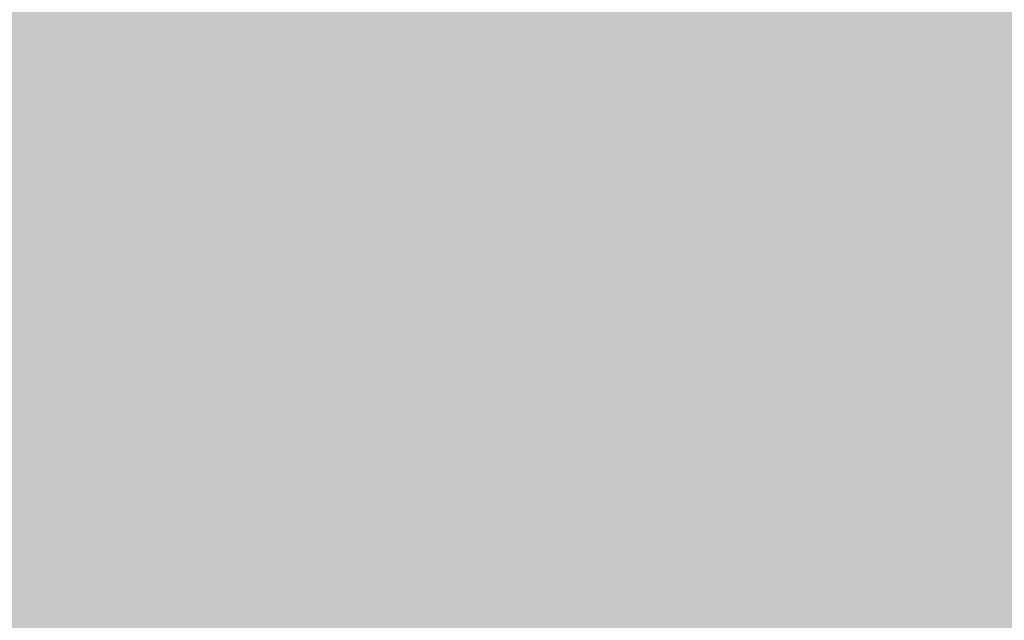
# Model space of a CAD drawing. Units: feet. Extents: x 3168 to 4724, y 827 to 1477.
# Tile 85 of 256: x 3274.148 to 3275.224, y 1098.344 to 1099.001. Entities that reach past the tile are written whole.
import ezdxf

# ---------------------------------------------------------------- set-up
doc = ezdxf.new("R2010")
doc.units = ezdxf.units.FT
doc.layers.add('A-ELEV', color=7, linetype='Continuous', lineweight=35)
doc.layers.add('A-ELEV-PATT', color=8, linetype='Continuous', lineweight=13)

msp = doc.modelspace()

# ---------------------------------------------------------------- hatches: boundary and pattern name
at = {"layer": 'A-ELEV-PATT'}
h = msp.add_hatch(color=256, dxfattribs=at)
h.dxf.hatch_style = 1
edge = h.paths.add_edge_path()
edge.add_ellipse((3552.9058, 979.2201), major_axis=(36.7449, 0), ratio=0.4848485, start_angle=0, end_angle=360)
edge = h.paths.add_edge_path()
edge.add_ellipse((3559.8916, 929.2523), major_axis=(36.7449, 0), ratio=0.4848485, start_angle=0, end_angle=360)
edge = h.paths.add_edge_path()
edge.add_line((3299.3168, 1198.6061), (3479.9167, 1198.6061))
edge.add_line((3479.9167, 1198.6061), (3479.9167, 1209.8686))
edge.add_spline(control_points=[(3479.9167, 1209.8686), (3464.3012, 1209.8686), (3448.6856, 1209.8686), (3410.9491, 1209.8686), (3388.8282, 1209.8686), (3355.6469, 1209.8686), (3344.5864, 1209.8686), (3327.9957, 1209.8686), (3322.4655, 1209.8686), (3314.1702, 1209.8686), (3311.4051, 1209.8686), (3307.2574, 1209.8686), (3305.8748, 1209.8686), (3303.801, 1209.8686), (3303.1097, 1209.8686), (3302.0728, 1209.8686), (3301.7272, 1209.8686), (3301.2087, 1209.8686), (3301.0359, 1209.8686), (3300.7767, 1209.8686), (3300.6903, 1209.8686), (3300.5606, 1209.8686), (3300.5174, 1209.8686), (3300.4526, 1209.8686), (3300.431, 1209.8686), (3300.3986, 1209.8686), (3300.3878, 1209.8686), (3300.3662, 1209.8686), (3300.3457, 1209.8686), (3300.3455, 1209.8686), (3300.3455, 1209.8686), (3300.3433, 1209.8686), (3300.3411, 1209.8686), (3300.3379, 1209.8686), (3300.3368, 1209.8686), (3300.3339, 1209.8686), (3300.3321, 1209.8686), (3300.3255, 1209.8686), (3300.3207, 1209.8686), (3300.3109, 1209.8686), (3300.306, 1209.8686), (3300.2905, 1209.8686), (3300.28, 1209.8686), (3300.2324, 1209.8688), (3300.1953, 1209.869), (3299.9511, 1209.8706), (3299.7448, 1209.8743), (3299.4368, 1209.8833), (3299.3344, 1209.8868), (3299.1811, 1209.8929), (3299.13, 1209.8951), (3298.6522, 1209.9168), (3298.2295, 1209.9457), (3297.6016, 1210.0024), (3297.3934, 1210.0235), (3297.0827, 1210.0583), (3296.9793, 1210.0705), (3296.293, 1210.1549), (3295.7181, 1210.2434), (3294.8687, 1210.3989), (3294.5877, 1210.4545), (3294.1693, 1210.5433), (3294.0304, 1210.5739), (3291.7071, 1211.1012), (3289.6536, 1211.8134), (3285.7763, 1213.564), (3283.9514, 1214.6035), (3280.5122, 1216.9801), (3278.8972, 1218.3176), (3276.3799, 1220.8295), (3275.416, 1221.9177), (3274.0393, 1223.7077), (3273.581, 1224.3495), (3273.1432, 1225.0163)], knot_values=[39.119033, 39.119033, 39.119033, 39.119033, 39.286353, 39.286353, 39.523379, 39.523379, 39.641892, 39.641892, 39.701148, 39.701148, 39.730777, 39.730777, 39.745591, 39.745591, 39.752998, 39.752998, 39.756701, 39.756701, 39.758553, 39.758553, 39.759479, 39.759479, 39.759942, 39.759942, 39.760173, 39.760173, 39.760289, 39.760289, 39.760405, 39.760405, 39.760463, 39.760463, 39.763389, 39.763389, 39.764851, 39.764851, 39.767304, 39.767304, 39.773825, 39.773825, 39.78057, 39.78057, 39.79477, 39.79477, 39.845194, 39.845194, 40.126715, 40.126715, 40.267476, 40.267476, 40.337856, 40.337856, 40.927023, 40.927023, 41.221606, 41.221606, 41.368898, 41.368898, 42.202622, 42.202622, 42.619485, 42.619485, 42.827916, 42.827916, 46.118323, 46.118323, 49.408731, 49.408731, 52.699139, 52.699139, 54.927489, 54.927489, 56.104228, 56.104228, 56.104228, 56.104228], weights=[1, 1, 1, 1, 1, 1, 1, 1, 1, 1, 1, 1, 1, 1, 1, 1, 1, 1, 1, 1, 1, 1, 1, 1, 1, 1, 1, 1, 1, 1, 1, 1, 1, 1, 1, 1, 1, 1, 1, 1, 1, 1, 1, 1, 1, 1, 1, 1, 1, 1, 1, 1, 1, 1, 1, 1, 1, 1, 1, 1, 1, 1, 1, 1, 1, 1, 1, 1, 1, 1, 1, 1, 1, 1], degree=3, periodic=0)
edge.add_line((3273.1432, 1225.0163), (3273.1432, 1099.0163))
edge.add_line((3273.1432, 1099.0163), (3299.3168, 1099.0163))
edge.add_line((3299.3168, 1099.0163), (3299.3168, 1198.6061))
edge = h.paths.add_edge_path()
edge.add_line((3304.7584, 1324.1581), (3479.9167, 1324.1581))
edge.add_line((3479.9167, 1324.1581), (3479.9167, 1335.7146))
edge.add_line((3479.9167, 1335.7146), (3269.1616, 1335.7146))
edge.add_spline(control_points=[(3269.1616, 1335.7146), (3264.0242, 1335.7146), (3258.3641, 1328.9582), (3259.2643, 1323.9003)], knot_values=[0, 0, 0, 0, 15.412191, 15.412191, 15.412191, 15.412191], degree=3, periodic=0)
edge.add_line((3259.2643, 1323.9003), (3265.5168, 1288.7691))
edge.add_line((3265.5168, 1288.7691), (3275.2651, 1261.5456))
edge.add_line((3275.2651, 1261.5456), (3304.7584, 1261.5456))
edge.add_line((3304.7584, 1261.5456), (3304.7584, 1324.1581))
h = msp.add_hatch(color=256, dxfattribs=at)
h.dxf.hatch_style = 1
h.paths.add_polyline_path([(3384.5252, 1099.0163), (3335.0292, 1099.0163), (3299.3168, 1099.0163), (3273.1432, 1099.0163), (3217.5654, 1099.0163), (3168.0693, 827.1163), (3335.0292, 827.1163)])

# ---------------------------------------------------------------- linework, layer by layer
at = {"layer": 'A-ELEV'}
msp.add_open_spline([(3808.5202, 1099.0163), (3808.5202, 1141.4132), (3808.5202, 1183.8102), (3808.5202, 1226.6353), (3808.5202, 1227.0636), (3808.5202, 1227.4918), (3811.4919, 1248.9947), (3814.4635, 1270.4975), (3817.4652, 1292.2176), (3817.4952, 1292.4348), (3817.5253, 1292.652), (3817.5728, 1310.1067), (3817.6203, 1327.5615), (3817.6679, 1345.0163), (3817.6679, 1345.458), (3817.6679, 1345.8996), (3817.6679, 1346.456), (3817.6679, 1346.5708), (3817.6679, 1346.7529), (3817.6679, 1346.8201), (3817.6679, 1346.9349), (3817.6679, 1346.9823), (3817.6679, 1347.0386), (3817.6679, 1347.0474), (3817.6679, 1347.0737), (3817.6679, 1347.0593), (3817.6679, 1347.0615), (3817.6679, 1347.0627), (3817.6679, 1347.066), (3817.6679, 1347.0683), (3817.6679, 1347.075), (3817.6679, 1347.0795), (3817.6678, 1347.0929), (3817.6678, 1347.1019), (3817.6678, 1347.1288), (3817.6677, 1347.1467), (3817.6674, 1347.2004), (3817.6672, 1347.2362), (3817.6661, 1347.3434), (3817.665, 1347.4147), (3817.6608, 1347.6281), (3817.6566, 1347.7697), (3817.64, 1348.1925), (3817.6235, 1348.4716), (3817.5591, 1349.3001), (3817.4961, 1349.8406), (3817.2554, 1351.4242), (3817.0263, 1352.4288), (3816.3069, 1354.8889), (3815.7437, 1356.2687), (3814.464, 1358.8192), (3813.7464, 1359.991), (3812.1958, 1362.1723), (3811.3622, 1363.1821), (3809.5888, 1365.069), (3808.6488, 1365.9461), (3806.6543, 1367.5796), (3805.5997, 1368.3362), (3803.3529, 1369.7223), (3802.1605, 1370.3524), (3799.6008, 1371.4536), (3798.2327, 1371.9255), (3795.2801, 1372.6346), (3793.6931, 1372.8721), (3791.8694, 1372.9265), (3791.7409, 1372.9292), (3791.3534, 1372.9341), (3791.0927, 1372.9329), (3790.3041, 1372.9151), (3789.7695, 1372.8842), (3789.2092, 1372.8302), (3789.1906, 1372.8284), (3789.1349, 1372.8229), (3789.0977, 1372.8191), (3789.0484, 1372.814), (3789.0364, 1372.8127), (3789.0003, 1372.8089), (3788.9761, 1372.8063), (3788.9494, 1372.8034), (3788.9468, 1372.8031), (3788.9426, 1372.8027), (3788.941, 1372.8025), (3788.9386, 1372.8022), (3788.9378, 1372.8021), (3788.9354, 1372.8019), (3788.8675, 1372.7944), (3788.7569, 1372.7822), (3788.7015, 1372.7761), (3788.5355, 1372.7579), (3788.4249, 1372.7457), (3788.0929, 1372.7092), (3787.8715, 1372.6848), (3787.2075, 1372.6118), (3786.7648, 1372.5631), (3785.4368, 1372.417), (3784.5515, 1372.3196), (3781.8954, 1372.0274), (3780.1247, 1371.8327), (3774.8126, 1371.2483), (3771.2713, 1370.8587), (3760.6471, 1369.69), (3753.5643, 1368.9109), (3732.316, 1366.5735), (3718.1504, 1365.0152), (3694.0068, 1362.3593), (3684.0287, 1361.2617), (3674.0506, 1360.1641), (3664.6007, 1360.1641), (3655.1508, 1360.1641), (3626.8011, 1360.1641), (3607.9013, 1360.1641), (3551.2019, 1360.1641), (3513.4023, 1360.1641), (3467.7252, 1360.1641), (3459.8476, 1360.1641), (3436.2149, 1360.1641), (3420.4597, 1360.1641), (3373.1943, 1360.1641), (3341.6839, 1360.1641), (3302.8482, 1360.1641), (3295.5227, 1360.1641), (3286.0383, 1360.1641), (3283.8794, 1360.1641), (3277.4026, 1360.1641), (3273.0848, 1360.1641), (3267.7329, 1360.1641), (3266.6988, 1360.1641), (3263.5965, 1360.1641), (3261.5284, 1360.1641), (3259.2369, 1360.1641), (3259.0137, 1360.1641), (3258.344, 1360.1641), (3257.8975, 1360.1641), (3257.431, 1360.1641), (3257.411, 1360.1641), (3257.3706, 1360.1641), (3257.3755, 1360.1641), (3257.3746, 1360.1641), (3257.3739, 1360.1641), (3257.372, 1360.1641), (3257.3706, 1360.1641), (3257.3667, 1360.1641), (3257.364, 1360.1641), (3257.3561, 1360.1641), (3257.3508, 1360.164), (3257.335, 1360.164), (3257.3244, 1360.164), (3257.2928, 1360.1639), (3257.2717, 1360.1638), (3257.2084, 1360.1634), (3257.1663, 1360.163), (3257.0402, 1360.1614), (3256.9563, 1360.1598), (3256.7055, 1360.1534), (3256.5392, 1360.147), (3256.0436, 1360.1219), (3255.7173, 1360.0971), (3254.7524, 1360.0005), (3254.128, 1359.9065), (3252.1801, 1359.5253), (3250.9416, 1359.144), (3248.6702, 1358.2433), (3247.6357, 1357.7238), (3245.7326, 1356.6035), (3244.8634, 1356.0021), (3243.2531, 1354.7429), (3242.512, 1354.0847), (3240.7511, 1352.3448), (3239.801, 1351.2296), (3238.0878, 1348.8724), (3237.3247, 1347.6304), (3235.9825, 1344.9716), (3235.4022, 1343.5549), (3234.5911, 1340.8155), (3234.3109, 1339.5435), (3233.9765, 1336.8026), (3233.9221, 1335.3309), (3234.1489, 1332.5913), (3234.3495, 1331.3672), (3234.7199, 1329.9994), (3234.7524, 1329.8834), (3234.8536, 1329.5348), (3234.9259, 1329.3017), (3235.0248, 1329.0026), (3235.0469, 1328.9369), (3235.0776, 1328.8472), (3235.0859, 1328.8232), (3235.1109, 1328.7511), (3235.1278, 1328.703), (3235.148, 1328.6462), (3235.1511, 1328.6376), (3235.1561, 1328.6235), (3235.1581, 1328.618), (3235.1602, 1328.612), (3235.1656, 1328.5969), (3235.1801, 1328.5565), (3235.1903, 1328.5281), (3235.2208, 1328.4429), (3235.2411, 1328.3862), (3235.3021, 1328.2159), (3235.3427, 1328.1023), (3235.4647, 1327.7617), (3235.546, 1327.5346), (3235.79, 1326.8534), (3235.9526, 1326.3992), (3236.4405, 1325.0367), (3236.7657, 1324.1284), (3237.7415, 1321.4034), (3238.392, 1319.5868), (3240.3435, 1314.1369), (3241.6445, 1310.5036), (3245.5476, 1299.6037), (3248.1496, 1292.3371), (3255.9557, 1270.5374), (3261.1598, 1256.0042), (3267.3876, 1238.612), (3268.4114, 1235.7529), (3269.5104, 1232.6839), (3269.5856, 1232.4739), (3269.7066, 1232.1359), (3269.7524, 1232.0079), (3269.8273, 1231.7987), (3269.8564, 1231.7176), (3269.9063, 1231.5781), (3269.9272, 1231.5198), (3269.9725, 1231.3934), (3269.9968, 1231.3254), (3270.0265, 1231.2425), (3270.0318, 1231.2277), (3270.0403, 1231.204), (3270.0392, 1231.207), (3270.0394, 1231.2066), (3270.0394, 1231.2064), (3270.0396, 1231.2058), (3270.0398, 1231.2055), (3270.0402, 1231.2043), (3270.0404, 1231.2036), (3270.0413, 1231.2013), (3270.0418, 1231.1998), (3270.0434, 1231.1953), (3270.0445, 1231.1922), (3270.0478, 1231.1832), (3270.0499, 1231.1771), (3270.0564, 1231.159), (3270.0608, 1231.147), (3270.0739, 1231.1108), (3270.0826, 1231.0867), (3270.1089, 1231.0144), (3270.1266, 1230.9663), (3270.1799, 1230.8225), (3270.2159, 1230.7269), (3270.3253, 1230.4415), (3270.4, 1230.2528), (3270.6292, 1229.6914), (3270.7889, 1229.3235), (3271.2865, 1228.2383), (3271.6431, 1227.5398), (3272.7759, 1225.5153), (3273.6142, 1224.2605), (3275.416, 1221.9177), (3276.3799, 1220.8295), (3278.8972, 1218.3176), (3280.5122, 1216.9801), (3283.9514, 1214.6035), (3285.7763, 1213.564), (3289.6536, 1211.8134), (3291.7071, 1211.1012), (3294.0304, 1210.5739), (3294.1693, 1210.5433), (3294.5877, 1210.4545), (3294.8687, 1210.3989), (3295.7181, 1210.2434), (3296.293, 1210.1549), (3296.9793, 1210.0705), (3297.0827, 1210.0583), (3297.3934, 1210.0235), (3297.6016, 1210.0024), (3298.2295, 1209.9457), (3298.6522, 1209.9168), (3299.13, 1209.8951), (3299.1811, 1209.8929), (3299.3344, 1209.8868), (3299.4368, 1209.8833), (3299.7448, 1209.8743), (3299.9511, 1209.8706), (3300.1953, 1209.869), (3300.2324, 1209.8688), (3300.28, 1209.8686), (3300.2905, 1209.8686), (3300.306, 1209.8686), (3300.3109, 1209.8686), (3300.3207, 1209.8686), (3300.3255, 1209.8686), (3300.3321, 1209.8686), (3300.3339, 1209.8686), (3300.3368, 1209.8686), (3300.3379, 1209.8686), (3300.3411, 1209.8686), (3300.3433, 1209.8686), (3300.3455, 1209.8686), (3300.3455, 1209.8686), (3300.3457, 1209.8686), (3300.3662, 1209.8686), (3300.3878, 1209.8686), (3300.3986, 1209.8686), (3300.431, 1209.8686), (3300.4526, 1209.8686), (3300.5174, 1209.8686), (3300.5606, 1209.8686), (3300.6903, 1209.8686), (3300.7767, 1209.8686), (3301.0359, 1209.8686), (3301.2087, 1209.8686), (3301.7272, 1209.8686), (3302.0728, 1209.8686), (3303.1097, 1209.8686), (3303.801, 1209.8686), (3305.8748, 1209.8686), (3307.2574, 1209.8686), (3311.4051, 1209.8686), (3314.1702, 1209.8686), (3322.4655, 1209.8686), (3327.9957, 1209.8686), (3344.5864, 1209.8686), (3355.6469, 1209.8686), (3388.8282, 1209.8686), (3410.9491, 1209.8686), (3477.3119, 1209.8686), (3521.5537, 1209.8686), (3566.8362, 1209.8686), (3567.8769, 1209.8686), (3570.999, 1209.8686), (3573.0804, 1209.8686), (3575.7814, 1209.8686), (3576.4009, 1209.8686), (3577.2958, 1209.8686), (3577.5712, 1209.8686), (3578.3971, 1209.8686), (3578.9478, 1209.8686), (3579.7565, 1209.8686), (3580.0145, 1209.8686), (3580.3427, 1209.8686), (3580.3269, 1209.8686), (3580.3272, 1209.8686), (3580.3273, 1209.8686), (3580.3278, 1209.8686), (3580.3281, 1209.8686), (3580.329, 1209.8686), (3580.3296, 1209.8686), (3580.3314, 1209.8686), (3580.3327, 1209.8686), (3580.3363, 1209.8686), (3580.3388, 1209.8686), (3580.3461, 1209.8686), (3580.351, 1209.8686), (3580.3657, 1209.8685), (3580.3754, 1209.8685), (3580.4048, 1209.8684), (3580.4244, 1209.8684), (3580.4832, 1209.8681), (3580.5224, 1209.8678), (3580.6404, 1209.8666), (3580.7192, 1209.8655), (3580.9563, 1209.8608), (3581.1152, 1209.8561), (3581.5942, 1209.8372), (3581.9164, 1209.8183), (3582.8899, 1209.7424), (3583.548, 1209.6662), (3585.5318, 1209.3606), (3586.8672, 1209.0539), (3589.4715, 1208.2525), (3590.7402, 1207.7579), (3591.9955, 1207.1588), (3592.0578, 1207.1287), (3592.2442, 1207.038), (3592.3677, 1206.9766), (3592.7353, 1206.7904), (3592.9768, 1206.6631), (3593.2445, 1206.5164), (3593.2747, 1206.4998), (3593.3651, 1206.4498), (3593.4251, 1206.4163), (3593.6043, 1206.3153), (3593.7227, 1206.2472), (3593.8572, 1206.1684), (3593.8744, 1206.1583), (3593.9257, 1206.128), (3593.9599, 1206.1078), (3594.0621, 1206.0469), (3594.1298, 1206.0061), (3594.2084, 1205.9582), (3594.2197, 1205.9513), (3594.2534, 1205.9307), (3594.2758, 1205.9169), (3594.343, 1205.8755), (3594.3876, 1205.8479), (3594.4336, 1205.819), (3594.4353, 1205.818), (3594.4402, 1205.8149), (3594.4435, 1205.8129), (3594.4471, 1205.8106), (3594.4475, 1205.8103), (3594.4487, 1205.8096), (3594.4495, 1205.8091), (3594.4504, 1205.8086), (3594.4505, 1205.8085), (3594.4506, 1205.8084), (3594.4674, 1205.7979), (3594.4933, 1205.7817), (3594.5062, 1205.7736), (3594.545, 1205.7492), (3594.5709, 1205.733), (3594.6485, 1205.6844), (3594.7002, 1205.652), (3594.8554, 1205.5547), (3594.9589, 1205.4898), (3595.2694, 1205.2953), (3595.4763, 1205.1656), (3596.0972, 1204.7765), (3596.5111, 1204.5171), (3597.7528, 1203.7388), (3598.5807, 1203.22), (3601.0642, 1201.6636), (3602.7198, 1200.6259), (3607.6868, 1197.513), (3610.9981, 1195.4377), (3620.932, 1189.2119), (3627.5546, 1185.0614), (3647.4225, 1172.6097), (3660.6678, 1164.3086), (3700.4035, 1139.4053), (3726.894, 1122.8031), (3757.2057, 1103.8061), (3761.027, 1101.4112), (3764.8482, 1099.0163), (3745.3283, 1099.0163), (3725.8083, 1099.0163), (3706.2884, 1099.0163), (3706.2884, 1108.4532), (3706.2884, 1117.8902), (3706.2884, 1127.3271), (3710.7508, 1127.3271), (3715.2131, 1127.3271), (3719.6755, 1127.3271)], degree=3, knots=[0, 0, 0, 0, 0.982037, 0.982037, 0.991957, 0.991957, 0.991957, 1.966522, 1.966522, 1.976367, 1.976367, 1.976367, 2.976367, 2.976367, 2.976367, 3.00169, 3.00169, 3.008272, 3.008272, 3.012129, 3.012129, 3.014851, 3.014851, 3.015353, 3.015353, 3.016359, 3.016359, 3.017365, 3.017365, 3.019376, 3.019376, 3.023398, 3.023398, 3.031442, 3.031442, 3.047531, 3.047531, 3.079708, 3.079708, 3.144063, 3.144063, 3.272772, 3.272772, 3.53019, 3.53019, 4.045026, 4.045026, 5.074698, 5.074698, 6.700878, 6.700878, 8.327058, 8.327058, 9.953238, 9.953238, 11.579418, 11.579418, 13.205598, 13.205598, 14.831778, 14.831778, 16.457958, 16.457958, 18.084138, 18.084138, 18.206872, 18.206872, 18.45234, 18.45234, 18.943275, 18.943275, 18.960093, 18.960093, 18.993729, 18.993729, 19.00461, 19.00461, 19.026374, 19.026374, 19.028737, 19.028737, 19.03018, 19.03018, 19.030897, 19.030897, 19.032332, 19.032332, 19.033766, 19.033766, 19.036636, 19.036636, 19.042374, 19.042374, 19.053851, 19.053851, 19.076805, 19.076805, 19.122714, 19.122714, 19.21453, 19.21453, 19.398163, 19.398163, 19.765429, 19.765429, 20.024128, 20.024128, 20.024128, 20.092031, 20.092031, 20.227836, 20.227836, 20.499446, 20.499446, 20.556051, 20.556051, 20.66926, 20.66926, 20.895678, 20.895678, 20.948316, 20.948316, 20.963829, 20.963829, 20.994855, 20.994855, 21.002285, 21.002285, 21.017146, 21.017146, 21.01875, 21.01875, 21.021959, 21.021959, 21.022102, 21.022102, 21.022249, 21.022249, 21.022708, 21.022708, 21.023627, 21.023627, 21.025464, 21.025464, 21.029138, 21.029138, 21.036486, 21.036486, 21.051183, 21.051183, 21.080575, 21.080575, 21.139361, 21.139361, 21.256932, 21.256932, 21.492073, 21.492073, 21.962356, 21.962356, 23.01002, 23.01002, 24.057684, 24.057684, 25.105348, 25.105348, 26.153011, 26.153011, 27.776787, 27.776787, 29.400562, 29.400562, 31.024337, 31.024337, 32.278801, 32.278801, 33.533265, 33.533265, 34.467568, 34.467568, 34.553971, 34.553971, 34.726776, 34.726776, 34.775309, 34.775309, 34.793079, 34.793079, 34.82862, 34.82862, 34.834979, 34.834979, 34.839039, 34.839039, 34.839411, 34.839411, 34.840285, 34.840285, 34.842034, 34.842034, 34.845531, 34.845531, 34.852525, 34.852525, 34.866512, 34.866512, 34.894488, 34.894488, 34.950439, 34.950439, 35.062342, 35.062342, 35.286147, 35.286147, 35.733758, 35.733758, 35.821815, 35.821815, 35.828283, 35.828283, 35.832225, 35.832225, 35.834724, 35.834724, 35.836521, 35.836521, 35.838617, 35.838617, 35.839073, 35.839073, 35.839345, 35.839345, 35.839617, 35.839617, 35.840161, 35.840161, 35.841249, 35.841249, 35.843425, 35.843425, 35.847778, 35.847778, 35.856482, 35.856482, 35.873891, 35.873891, 35.908709, 35.908709, 35.978345, 35.978345, 36.117617, 36.117617, 36.396161, 36.396161, 36.953248, 36.953248, 38.067423, 38.067423, 40.295772, 40.295772, 42.524122, 42.524122, 45.81453, 45.81453, 49.104937, 49.104937, 52.395345, 52.395345, 52.603776, 52.603776, 53.020639, 53.020639, 53.854363, 53.854363, 54.001655, 54.001655, 54.296238, 54.296238, 54.885405, 54.885405, 54.955785, 54.955785, 55.096546, 55.096546, 55.378067, 55.378067, 55.42849, 55.42849, 55.442691, 55.442691, 55.449436, 55.449436, 55.455957, 55.455957, 55.458409, 55.458409, 55.459872, 55.459872, 55.462798, 55.462798, 55.462856, 55.462856, 55.462972, 55.462972, 55.463088, 55.463088, 55.463319, 55.463319, 55.463782, 55.463782, 55.464708, 55.464708, 55.46656, 55.46656, 55.470263, 55.470263, 55.47767, 55.47767, 55.492484, 55.492484, 55.522112, 55.522112, 55.581369, 55.581369, 55.699882, 55.699882, 55.936907, 55.936907, 56.410959, 56.410959, 56.42211, 56.42211, 56.444413, 56.444413, 56.451051, 56.451051, 56.454001, 56.454001, 56.459901, 56.459901, 56.462666, 56.462666, 56.463418, 56.463418, 56.464171, 56.464171, 56.465675, 56.465675, 56.468684, 56.468684, 56.474702, 56.474702, 56.486738, 56.486738, 56.51081, 56.51081, 56.558955, 56.558955, 56.655243, 56.655243, 56.847821, 56.847821, 57.232975, 57.232975, 58.003284, 58.003284, 59.543901, 59.543901, 62.625137, 62.625137, 68.787607, 68.787607, 74.950078, 74.950078, 75.27336, 75.27336, 75.919923, 75.919923, 77.213051, 77.213051, 77.377769, 77.377769, 77.707206, 77.707206, 78.366079, 78.366079, 78.462532, 78.462532, 78.655436, 78.655436, 79.041245, 79.041245, 79.105735, 79.105735, 79.234714, 79.234714, 79.492672, 79.492672, 79.502197, 79.502197, 79.521249, 79.521249, 79.523534, 79.523534, 79.528103, 79.528103, 79.528682, 79.528682, 79.528885, 79.528885, 79.529089, 79.529089, 79.529495, 79.529495, 79.530308, 79.530308, 79.531935, 79.531935, 79.535187, 79.535187, 79.541693, 79.541693, 79.554704, 79.554704, 79.580725, 79.580725, 79.632769, 79.632769, 79.736856, 79.736856, 79.94503, 79.94503, 80.361377, 80.361377, 80.421435, 80.421435, 80.421435, 81.421435, 81.421435, 81.421435, 82.421435, 82.421435, 82.421435, 83.421435, 83.421435, 83.421435, 83.421435], dxfattribs=at)

doc.saveas('drawing.dxf')
